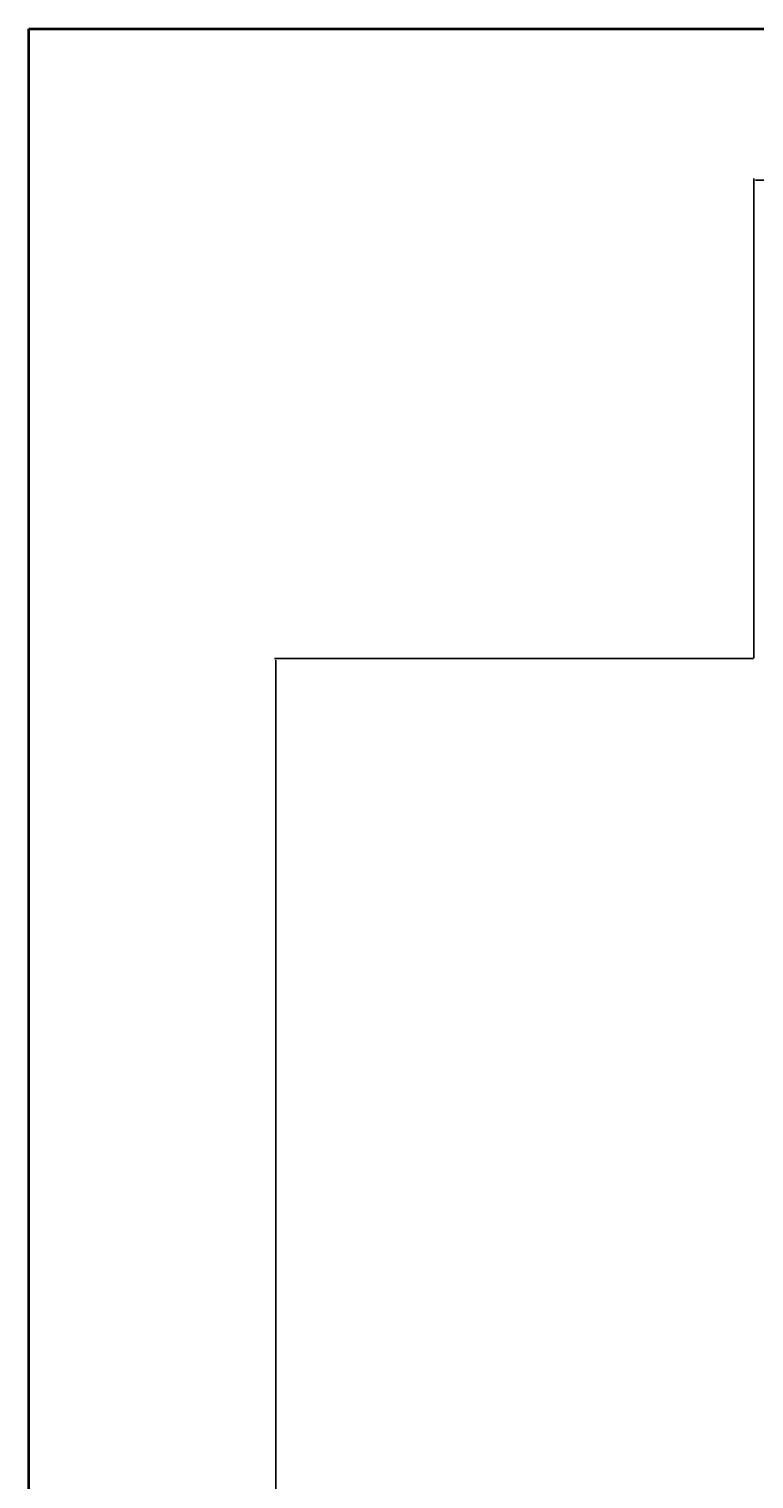
# Model space of a CAD drawing. Units: inches. Extents: x 1088 to 1703, y 668 to 1875.
# Tile 14 of 45: x 1088 to 1170, y 1711 to 1875. Entities that reach past the tile are written whole.
import ezdxf

# ---------------------------------------------------------------- set-up
doc = ezdxf.new("R2010")
doc.units = ezdxf.units.IN
doc.layers.add('A-ANNO-DIMS', color=2, linetype='Continuous', lineweight=18)
doc.layers.add('A-ANNO-TTLB', color=7, linetype='Continuous', lineweight=35)
doc.styles.get("Standard").update_dxf_attribs({"font": 'arial.ttf'})
doc.dimstyles.get("Standard").update_dxf_attribs({"dimtxt": 0.18, "dimasz": 0.18, "dimexe": 0.18, "dimexo": 0.0625, "dimgap": 0.09, "dimtad": 0, "dimtih": 1, "dimtoh": 1, "dimdec": 4, "dimzin": 0, "dimdsep": 46, "dimtxsty": 'Standard', "dimcen": 0.09, "dimadec": 0, "dimazin": 0, "dimtfac": 1, "dimtdec": 4, "dimtofl": 0, "dimtmove": 0, "dimatfit": 3, "dimfxl": 1, "dimtolj": 1, "dimtzin": 0, "dimarcsym": 0})

# ---------------------------------------------------------------- blocks, each defined once
blk = doc.blocks.new('*D28')
at = {"layer": 'A-ANNO-DIMS', "color": 0, "lineweight": -2, "transparency": 16777216}
for p, q in [((1170.34, 1803.62), (1170.34, 1857.79)), ((1170.52, 1857.61), (1408.15, 1857.61)), ((1646.56, 1857.61), (1408.94, 1857.61)), ((1646.74, 1745.55), (1646.74, 1857.79))]:
    blk.add_line(p, q, dxfattribs=at)
at = {"layer": 'A-ANNO-DIMS', "color": 0, "transparency": 16777216}
for points in [[(1170.52, 1857.64), (1170.52, 1857.58), (1170.34, 1857.61)], [(1646.56, 1857.64), (1646.56, 1857.58), (1646.74, 1857.61)]]:
    blk.add_solid(points, dxfattribs=at)
at = {"layer": 'Defpoints', "color": 0, "transparency": 16777216}
for p in [(1646.74, 1857.61), (1170.34, 1803.56), (1646.74, 1745.49)]:
    blk.add_point(p, dxfattribs=at)
at = {"layer": 'A-ANNO-DIMS', "color": 0, "transparency": 16777216, "insert": (1408.54, 1857.61), "char_height": 0.18, "attachment_point": 5}
blk.add_mtext('\\A1;476.4', dxfattribs=at)
blk = doc.blocks.new('*D29')
at = {"layer": 'A-ANNO-DIMS', "color": 0, "lineweight": -2, "transparency": 16777216}
for p, q in [((1170.28, 1803.56), (1116.11, 1803.56)), ((1116.29, 1803.38), (1116.29, 1291.85)), ((1116.29, 779.96), (1116.29, 1291.49)), ((1170.28, 779.78), (1116.11, 779.78))]:
    blk.add_line(p, q, dxfattribs=at)
at = {"layer": 'A-ANNO-DIMS', "color": 0, "transparency": 16777216}
for points in [[(1116.26, 1803.38), (1116.32, 1803.38), (1116.29, 1803.56)], [(1116.26, 779.96), (1116.32, 779.96), (1116.29, 779.78)]]:
    blk.add_solid(points, dxfattribs=at)
at = {"layer": 'Defpoints', "color": 0, "transparency": 16777216}
for p in [(1116.29, 1803.56), (1170.34, 1803.56), (1170.34, 779.78)]:
    blk.add_point(p, dxfattribs=at)
at = {"layer": 'A-ANNO-DIMS', "color": 0, "transparency": 16777216, "insert": (1116.29, 1291.67), "char_height": 0.18, "attachment_point": 5}
blk.add_mtext('\\A1;1023.8', dxfattribs=at)

msp = doc.modelspace()

# ---------------------------------------------------------------- linework, layer by layer
at = {"layer": 'A-ANNO-TTLB'}
msp.add_lwpolyline([(1088.369, 1874.677), (1703.181, 1874.677), (1703.181, 667.947), (1088.369, 667.947)], close=True, dxfattribs=at)

# ---------------------------------------------------------------- dimensions: what is measured, and where the dimension line sits
at = {"layer": 'A-ANNO-DIMS'}
dim = msp.add_linear_dim(base=(1646.743, 1857.608), p1=(1170.345, 1803.558), p2=(1646.743, 1745.49), dimstyle='Standard', override={"dimdec": 1, "dimlfac": 1, "dimrnd": 0, "dimzin": 0, "dimdsep": 46, "dimlunit": 2}, dxfattribs=at)
dim.commit()
dim.dimension.update_dxf_attribs({"geometry": '*D28', "text_midpoint": (1408.544, 1857.608)})
dim = msp.add_linear_dim(base=(1116.295, 1803.558), p1=(1170.345, 779.779), p2=(1170.345, 1803.558), angle=90, dimstyle='Standard', override={"dimdec": 1, "dimlfac": 1, "dimrnd": 0, "dimzin": 0, "dimdsep": 46, "dimlunit": 2}, dxfattribs=at)
dim.commit()
dim.dimension.update_dxf_attribs({"geometry": '*D29', "text_midpoint": (1116.295, 1291.669)})

doc.saveas('drawing.dxf')
